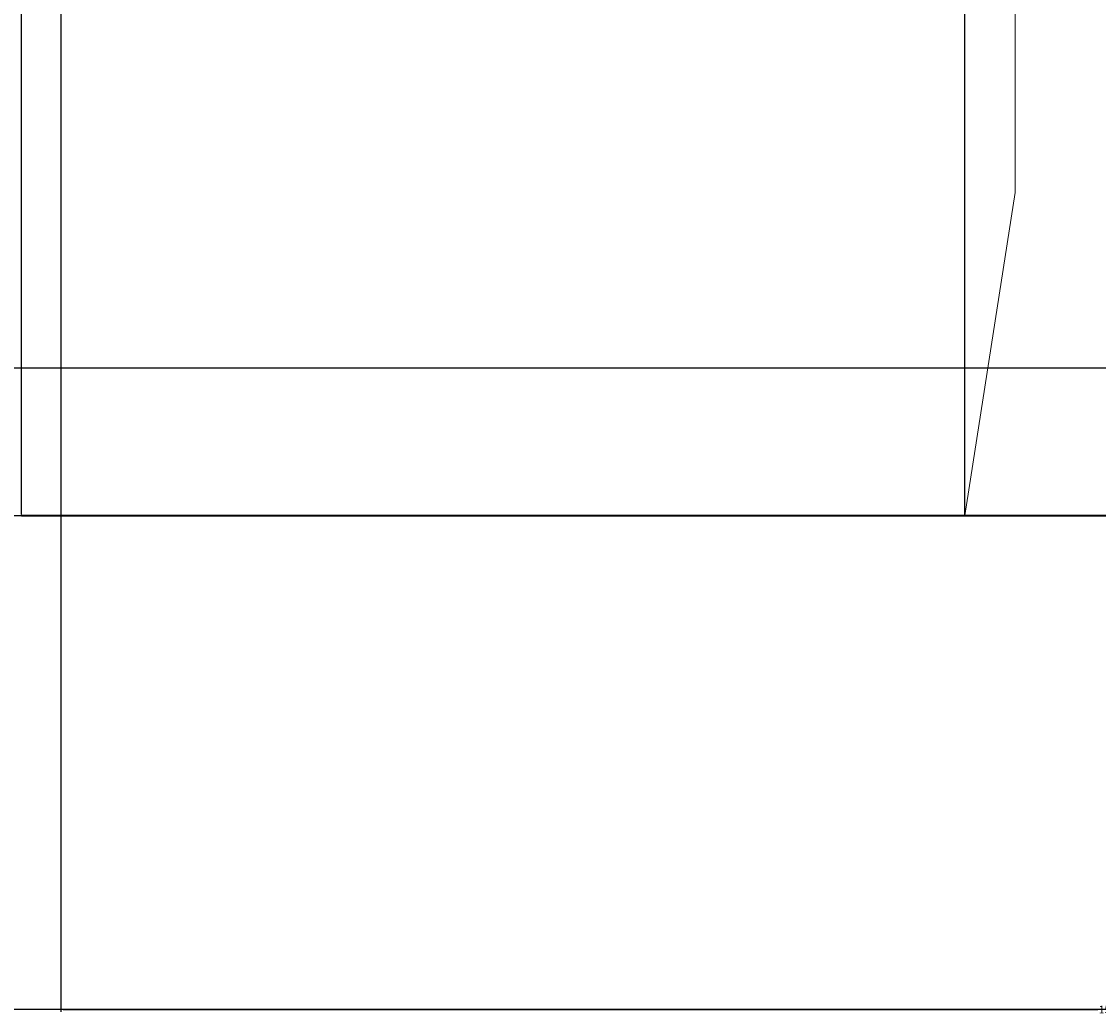
# Model space of a CAD drawing. Units: inches. Extents: x -26 to 776, y -22 to 650.
# Tile 41 of 62: x 426 to 506, y -22 to 52. Entities that reach past the tile are written whole.
import ezdxf

# ---------------------------------------------------------------- set-up
doc = ezdxf.new("R2010")
doc.units = ezdxf.units.IN
doc.header["$MEASUREMENT"] = 0
for name, color, linetype, lineweight in [('A-ANNO-DIMS', 2, 'Continuous', 18), ('C-TOPO', 7, 'Continuous', 35), ('L-PLNT-TREE', 94, 'Continuous', 18)]:
    doc.layers.add(name, color=color, linetype=linetype, lineweight=lineweight)
doc.styles.get("Standard").update_dxf_attribs({"font": 'arial.ttf'})
doc.dimstyles.get("Standard").update_dxf_attribs({"dimtxt": 0.5625, "dimasz": 0.18, "dimexe": 0.18, "dimexo": 0.0625, "dimgap": 0.09, "dimtad": 0, "dimtih": 1, "dimtoh": 1, "dimdec": 4, "dimzin": 0, "dimdsep": 46, "dimlunit": 4, "dimtxsty": 'Standard', "dimcen": 0.09, "dimadec": 0, "dimazin": 0, "dimtfac": 1, "dimtdec": 4, "dimtofl": 0, "dimtmove": 0, "dimatfit": 3, "dimfxl": 1, "dimtolj": 1, "dimtzin": 0, "dimarcsym": 0})

# ---------------------------------------------------------------- blocks, each defined once
blk = doc.blocks.new('Tree - type 2 deciduous elevation')
blk.add_lwpolyline([(-6.813, 23.669), (-6.813, 11.669), (-8.627, 0)])
blk = doc.blocks.new('*D13')
at = {"layer": 'A-ANNO-DIMS', "color": 0, "lineweight": -2, "transparency": 16777216}
for p, q in [((738.75, 50.786), (738.75, -21.315)), ((11.107, 15.42), (11.107, -21.315)), ((11.287, -21.135), (373.892, -21.135)), ((738.57, -21.135), (375.965, -21.135))]:
    blk.add_line(p, q, dxfattribs=at)
at = {"layer": 'A-ANNO-DIMS', "color": 0, "transparency": 16777216}
for points in [[(11.287, -21.105), (11.287, -21.165), (11.107, -21.135)], [(738.57, -21.105), (738.57, -21.165), (738.75, -21.135)]]:
    blk.add_solid(points, dxfattribs=at)
at = {"layer": 'Defpoints', "color": 0, "transparency": 16777216}
for p in [(738.75, 50.848), (11.107, 15.482), (738.75, -21.135)]:
    blk.add_point(p, dxfattribs=at)
at = {"layer": 'A-ANNO-DIMS', "color": 0, "transparency": 16777216, "insert": (374.929, -21.135), "char_height": 0.5625, "attachment_point": 5}
blk.add_mtext('\\A1;727.6', dxfattribs=at)
blk = doc.blocks.new('*D20')
at = {"layer": 'A-ANNO-DIMS', "color": 0, "lineweight": -2, "transparency": 16777216}
for p, q in [((425.806, 455.472), (775.335, 455.472)), ((775.155, 455.292), (775.155, 235.854)), ((775.155, 15.662), (775.155, 235.1)), ((425.806, 15.482), (775.335, 15.482))]:
    blk.add_line(p, q, dxfattribs=at)
at = {"layer": 'A-ANNO-DIMS', "color": 0, "transparency": 16777216}
for points in [[(775.125, 455.292), (775.185, 455.292), (775.155, 455.472)], [(775.125, 15.662), (775.185, 15.662), (775.155, 15.482)]]:
    blk.add_solid(points, dxfattribs=at)
at = {"layer": 'Defpoints', "color": 0, "transparency": 16777216}
for p in [(425.743, 455.472), (775.155, 455.472), (425.743, 15.482)]:
    blk.add_point(p, dxfattribs=at)
at = {"layer": 'A-ANNO-DIMS', "color": 0, "transparency": 16777216, "insert": (775.155, 235.477), "char_height": 0.5625, "attachment_point": 5}
blk.add_mtext('\\A1;440', dxfattribs=at)
blk = doc.blocks.new('*D30')
at = {"layer": 'A-ANNO-DIMS', "color": 0, "lineweight": -2, "transparency": 16777216}
for p, q in [((280.68, 144.836), (775.335, 144.836)), ((775.155, 144.656), (775.155, 86.007)), ((775.155, 26.604), (775.155, 85.253)), ((280.68, 26.424), (775.335, 26.424))]:
    blk.add_line(p, q, dxfattribs=at)
at = {"layer": 'A-ANNO-DIMS', "color": 0, "transparency": 16777216}
for points in [[(775.125, 144.656), (775.185, 144.656), (775.155, 144.836)], [(775.125, 26.604), (775.185, 26.604), (775.155, 26.424)]]:
    blk.add_solid(points, dxfattribs=at)
at = {"layer": 'Defpoints', "color": 0, "transparency": 16777216}
for p in [(280.617, 144.836), (775.155, 144.836), (280.617, 26.424)]:
    blk.add_point(p, dxfattribs=at)
at = {"layer": 'A-ANNO-DIMS', "color": 0, "transparency": 16777216, "insert": (775.155, 85.63), "char_height": 0.5625, "attachment_point": 5}
blk.add_mtext('\\A1;118.41', dxfattribs=at)
blk = doc.blocks.new('*D38')
at = {"layer": 'A-ANNO-DIMS', "color": 0, "lineweight": -2, "transparency": 16777216}
for p, q in [((280.68, 26.424), (775.335, 26.424)), ((775.155, 26.244), (775.155, 21.33)), ((775.155, 15.662), (775.155, 20.576)), ((289.305, 15.482), (775.335, 15.482))]:
    blk.add_line(p, q, dxfattribs=at)
at = {"layer": 'A-ANNO-DIMS', "color": 0, "transparency": 16777216}
for points in [[(775.125, 26.244), (775.185, 26.244), (775.155, 26.424)], [(775.125, 15.662), (775.185, 15.662), (775.155, 15.482)]]:
    blk.add_solid(points, dxfattribs=at)
at = {"layer": 'Defpoints', "color": 0, "transparency": 16777216}
for p in [(280.617, 26.424), (775.155, 26.424), (289.242, 15.482)]:
    blk.add_point(p, dxfattribs=at)
at = {"layer": 'A-ANNO-DIMS', "color": 0, "transparency": 16777216, "insert": (775.155, 20.953), "char_height": 0.5625, "attachment_point": 5}
blk.add_mtext('\\A1;10.942', dxfattribs=at)
blk = doc.blocks.new('*D39')
at = {"layer": 'A-ANNO-DIMS', "color": 0, "lineweight": -2, "transparency": 16777216}
for p, q in [((289.242, 15.545), (289.242, 649.856)), ((289.422, 649.676), (356.478, 649.676)), ((425.563, 649.676), (358.508, 649.676)), ((425.743, 15.545), (425.743, 649.856))]:
    blk.add_line(p, q, dxfattribs=at)
at = {"layer": 'A-ANNO-DIMS', "color": 0, "transparency": 16777216}
for points in [[(289.422, 649.706), (289.422, 649.646), (289.242, 649.676)], [(425.563, 649.706), (425.563, 649.646), (425.743, 649.676)]]:
    blk.add_solid(points, dxfattribs=at)
at = {"layer": 'Defpoints', "color": 0, "transparency": 16777216}
for p in [(425.743, 649.676), (289.242, 15.482), (425.743, 15.482)]:
    blk.add_point(p, dxfattribs=at)
at = {"layer": 'A-ANNO-DIMS', "color": 0, "transparency": 16777216, "insert": (357.493, 649.676), "char_height": 0.5625, "attachment_point": 5}
blk.add_mtext('\\A1;136.5', dxfattribs=at)
blk = doc.blocks.new('*D40')
at = {"layer": 'A-ANNO-DIMS', "color": 0, "lineweight": -2, "transparency": 16777216}
for p, q in [((425.743, 15.545), (425.743, 649.856)), ((425.923, 649.676), (459.646, 649.676)), ((495.451, 649.676), (461.728, 649.676)), ((495.631, 15.545), (495.631, 649.856))]:
    blk.add_line(p, q, dxfattribs=at)
at = {"layer": 'A-ANNO-DIMS', "color": 0, "transparency": 16777216}
for points in [[(425.923, 649.706), (425.923, 649.646), (425.743, 649.676)], [(495.451, 649.706), (495.451, 649.646), (495.631, 649.676)]]:
    blk.add_solid(points, dxfattribs=at)
at = {"layer": 'Defpoints', "color": 0, "transparency": 16777216}
for p in [(495.631, 649.676), (425.743, 15.482), (495.631, 15.482)]:
    blk.add_point(p, dxfattribs=at)
at = {"layer": 'A-ANNO-DIMS', "color": 0, "transparency": 16777216, "insert": (460.687, 649.676), "char_height": 0.5625, "attachment_point": 5}
blk.add_mtext('\\A1;69.89', dxfattribs=at)
blk = doc.blocks.new('*D47')
at = {"layer": 'A-ANNO-DIMS', "color": 0, "lineweight": -2, "transparency": 16777216}
for p, q in [((584.343, 199.901), (584.343, -21.315)), ((428.648, 180.243), (428.648, -21.315)), ((428.828, -21.135), (505.483, -21.135)), ((584.163, -21.135), (507.508, -21.135))]:
    blk.add_line(p, q, dxfattribs=at)
at = {"layer": 'A-ANNO-DIMS', "color": 0, "transparency": 16777216}
for points in [[(428.828, -21.105), (428.828, -21.165), (428.648, -21.135)], [(584.163, -21.105), (584.163, -21.165), (584.343, -21.135)]]:
    blk.add_solid(points, dxfattribs=at)
at = {"layer": 'Defpoints', "color": 0, "transparency": 16777216}
for p in [(584.343, 199.963), (428.648, 180.305), (584.343, -21.135)]:
    blk.add_point(p, dxfattribs=at)
at = {"layer": 'A-ANNO-DIMS', "color": 0, "transparency": 16777216, "insert": (506.496, -21.135), "char_height": 0.5625, "attachment_point": 5}
blk.add_mtext('\\A1;155.7', dxfattribs=at)

msp = doc.modelspace()

# ---------------------------------------------------------------- linework, layer by layer
at = {"layer": 'C-TOPO'}
msp.add_line((425.7434, 15.4824), (677.9037, 15.4824), dxfattribs=at)

# ---------------------------------------------------------------- block references
at = {"layer": 'L-PLNT-TREE', "xscale": 2.050905272406618, "yscale": 2.050905272406618, "zscale": 2.050905272406618}
msp.add_blockref('Tree - type 2 deciduous elevation', (513.3241, 15.4824), dxfattribs=at)

# ---------------------------------------------------------------- dimensions: what is measured, and where the dimension line sits
at = {"layer": 'A-ANNO-DIMS'}
for base, p1, p2, override, picture, middle in [((425.7434, 649.6763), (289.2424, 15.4824), (425.7434, 15.4824), {"dimdec": 1, "dimlfac": 1, "dimrnd": 0, "dimzin": 0, "dimdsep": 46, "dimlunit": 2}, '*D39', (357.4929, 649.6763)), ((495.6309, 649.6763), (425.7434, 15.4824), (495.6309, 15.4824), {"dimdec": 2, "dimlfac": 1, "dimrnd": 0, "dimzin": 0, "dimdsep": 46, "dimlunit": 2}, '*D40', (460.6872, 649.6763)), ((584.3428, -21.1349), (428.6484, 180.3054), (584.3428, 199.9634), {"dimdec": 1, "dimlfac": 1, "dimrnd": 0, "dimzin": 0, "dimdsep": 46, "dimlunit": 2}, '*D47', (506.4956, -21.1349)), ((738.7503, -21.1349), (11.1074, 15.4824), (738.7503, 50.8482), {"dimdec": 1, "dimlfac": 1, "dimrnd": 0, "dimzin": 0, "dimdsep": 46, "dimlunit": 2}, '*D13', (374.9289, -21.1349))]:
    dim = msp.add_linear_dim(base=base, p1=p1, p2=p2, dimstyle='Standard', override=override, dxfattribs=at)
    dim.commit()
    dim.dimension.update_dxf_attribs({"geometry": picture, "text_midpoint": middle})
for base, p1, p2, override, picture, middle in [((775.1553, 455.4717), (425.7434, 15.4824), (425.7434, 455.4717), {"dimdec": 0, "dimlfac": 1, "dimrnd": 0, "dimzin": 0, "dimdsep": 46, "dimlunit": 2}, '*D20', (775.1553, 235.477)), ((775.1553, 144.8359), (280.6173, 26.4239), (280.6173, 144.8359), {"dimdec": 2, "dimlfac": 1, "dimrnd": 0, "dimzin": 0, "dimdsep": 46, "dimlunit": 2}, '*D30', (775.1553, 85.6299)), ((775.15535, 26.4239), (289.24236, 15.48237), (280.61732, 26.4239), {"dimdec": 3, "dimlfac": 1, "dimrnd": 0, "dimzin": 0, "dimdsep": 46, "dimlunit": 2}, '*D38', (775.15535, 20.95313))]:
    dim = msp.add_linear_dim(base=base, p1=p1, p2=p2, angle=90, dimstyle='Standard', override=override, dxfattribs=at)
    dim.commit()
    dim.dimension.update_dxf_attribs({"geometry": picture, "text_midpoint": middle})

doc.saveas('drawing.dxf')
